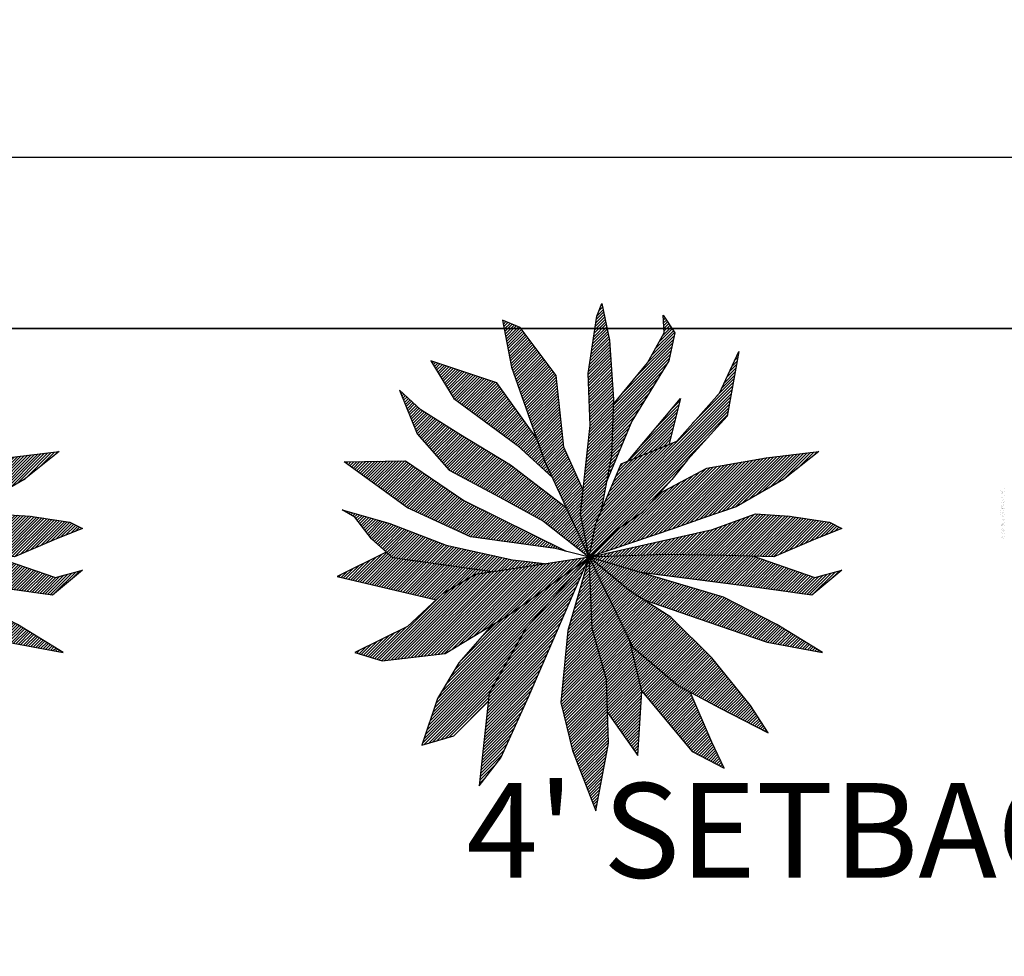
# Model space of a CAD drawing. Units: inches. Extents: x 1986 to 21484, y -1816 to 2016.
# Tile 10 of 85: x 2076 to 2149, y 1854 to 1924. Entities that reach past the tile are written whole.
import ezdxf

# ---------------------------------------------------------------- set-up
doc = ezdxf.new("R2010")
doc.units = ezdxf.units.IN
for name, color, linetype, lineweight in [('A-ANNO-DIMS', 2, 'Continuous', 18), ('A-ANNO-TEXT', 7, 'Continuous', 18), ('C-PROP', 7, 'Continuous', 35), ('L-PLNT', 84, 'Continuous', 13), ('vfolhas', 114, 'Continuous', 5)]:
    doc.layers.add(name, color=color, linetype=linetype, lineweight=lineweight)
for name, color, linetype in [('vfolha', 72, 'Continuous'), ('vfolha2', 110, 'Continuous'), ('vfolhas2', 102, 'Continuous')]:
    doc.layers.add(name, color=color, linetype=linetype)
doc.styles.get("Standard").update_dxf_attribs({"font": 'arial.ttf'})
doc.dimstyles.new('ISO-25', dxfattribs={"dimtxt": 8, "dimasz": 2.5, "dimexe": 1.25, "dimexo": 0.625, "dimtad": 1, "dimdec": 1, "dimlunit": 3, "dimtxsty": 'Standard', "dimcen": 2.5, "dimadec": 0, "dimazin": 0, "dimtfac": 1, "dimtdec": 1, "dimtmove": 0, "dimatfit": 3, "dimfxl": 1, "dimarcsym": 0})
pattern_1 = [(45, (-2446.5133113, 50.986076), (-0.004419417382, 0.004419417382), [])]

# ---------------------------------------------------------------- blocks, each defined once
blk = doc.blocks.new('*D1')
at = {"layer": 'A-ANNO-DIMS', "color": 0, "lineweight": -2, "transparency": 16777216}
for p, q in [((2042.312, 1901.377), (2042.312, 1914.655)), ((2402.312, 1901.377), (2402.312, 1914.655)), ((2044.812, 1913.405), (2399.812, 1913.405))]:
    blk.add_line(p, q, dxfattribs=at)
at = {"layer": 'A-ANNO-DIMS', "color": 0, "transparency": 16777216}
for points in [[(2044.812, 1913.821), (2044.812, 1912.988), (2042.312, 1913.405)], [(2399.812, 1913.821), (2399.812, 1912.988), (2402.312, 1913.405)]]:
    blk.add_solid(points, dxfattribs=at)
at = {"layer": 'Defpoints', "color": 0, "transparency": 16777216}
for p in [(2402.312, 1913.405), (2042.312, 1900.752), (2402.312, 1900.752)]:
    blk.add_point(p, dxfattribs=at)
at = {"layer": 'A-ANNO-DIMS', "color": 0, "transparency": 16777216, "insert": (2222.312, 1918.117), "char_height": 8, "attachment_point": 5}
blk.add_mtext("30'", dxfattribs=at)
blk = doc.blocks.new('arbusto_PB_verde_grande')
at = {"layer": 'vfolha2'}
h = blk.add_hatch(dxfattribs=at)
h.set_pattern_fill('ANSI31', color=256, scale=0.05, style=0)
h.set_pattern_definition(pattern_1)
h.paths.add_polyline_path([(0.0294, 0.3565), (0.0003, 0.0905), (0.0263, -0.0393), (0.047, 0.0623), (0.0619, 0.0973), (0.0937, 0.2657), (0.0996, 0.4347), (0.0879, 0.6131), (0.0645, 0.7227), (0.0499, 0.6851), (0.0236, 0.5129)])
h.paths.add_polyline_path([(0.3011, 0.4379), (0.1423, 0.2487), (0.2669, 0.3002)])
h.paths.add_polyline_path([(0.38, 0.2282), (0.237, 0.1519), (0.1843, 0.0936), (0.1112, 0.0436), (0.0263, -0.0393), (0.2806, 0.0467), (0.3683, 0.078), (0.4676, 0.1124), (0.6107, 0.1938), (0.7159, 0.2782), (0.5581, 0.2595)])
h.paths.add_polyline_path([(0.561, -0.2944), (0.7275, -0.3257), (0.5902, -0.2412), (0.4296, -0.1598), (0.0263, -0.0393), (0.1492, -0.1411), (0.1884, -0.166), (0.415, -0.2444)])
h.paths.add_polyline_path([(-0.2743, -0.4478), (-0.3035, -0.7263), (-0.2392, -0.6417), (-0.1546, -0.4572), (0.0263, -0.0393), (-0.1633, -0.2538)])
h.paths.add_polyline_path([(-0.5196, -0.2474), (-0.6774, -0.3257), (-0.5956, -0.3507), (-0.4057, -0.3288), (-0.2101, -0.21), (0.0263, -0.0393), (-0.1487, -0.0659), (-0.3152, -0.091), (-0.4145, -0.1505)])
h.paths.add_polyline_path([(-0.5255, 0.2501), (-0.7095, 0.247), (-0.5196, 0.1093), (-0.3298, 0.0217), (-0.0757, -0.0128), (-0.0423, -0.0215), (-0.3502, 0.1312)])
h = blk.add_hatch(dxfattribs=at)
h.set_pattern_fill('ANSI31', color=256, scale=0.05, style=0)
h.set_pattern_definition(pattern_1)
h.paths.add_polyline_path([(-0.1896, 0.297), (-0.0855, 0.2019), (-0.1078, 0.2501), (-0.132, 0.3187), (-0.251, 0.4848), (-0.4495, 0.5505), (-0.3795, 0.4379)])
h.paths.add_polyline_path([(0.0791, -0.4071), (0.0821, -0.5063), (0.1726, -0.6355), (0.1843, -0.4415), (0.149, -0.2918), (0.0263, -0.0393), (0.0353, -0.2538)])
at = {"layer": 'vfolhas'}
h = blk.add_hatch(dxfattribs=at)
h.set_pattern_fill('ANSI31', color=256, scale=0.05, style=0)
h.set_pattern_definition(pattern_1)
h.paths.add_polyline_path([(-0.0728, 0.5067), (-0.1808, 0.6506), (-0.2334, 0.6725), (-0.2071, 0.5318), (-0.1078, 0.2501), (0.0263, -0.0393), (0.0003, 0.0905), (0.0082, 0.1624), (-0.0494, 0.2908)])
h.paths.add_polyline_path([(0.099, 0.4193), (0.0937, 0.2657), (0.0791, 0.1881), (0.1551, 0.369), (0.2661, 0.5505), (0.2836, 0.635), (0.2485, 0.6882), (0.2514, 0.635), (0.2018, 0.5443)])
h.paths.add_polyline_path([(0.1229, 0.2407), (0.047, 0.0623), (0.0263, -0.0393), (0.1112, 0.0436), (0.1843, 0.0936), (0.2748, 0.1938), (0.3215, 0.2532), (0.4413, 0.3847), (0.4763, 0.5787), (0.4179, 0.4535), (0.2894, 0.3095)])
h.paths.add_polyline_path([(0.5815, -0.0378), (0.7071, 0.0154), (0.7859, 0.0467), (0.748, 0.0655), (0.6282, 0.0842), (0.526, 0.0905), (0.3974, 0.0436), (0.0263, -0.0393), (0.2573, -0.0315), (0.4383, -0.0347)])
h.paths.add_polyline_path([(0.5202, -0.0365), (0.4383, -0.0347), (0.2573, -0.0315), (0.0263, -0.0393), (0.1796, -0.0852), (0.5377, -0.1317), (0.6954, -0.1536), (0.7859, -0.0785), (0.7041, -0.1004)])
h.paths.add_polyline_path([(0.2719, -0.2193), (0.1492, -0.1411), (0.0263, -0.0393), (0.1579, -0.3101), (0.2952, -0.4258), (0.4179, -0.4916), (0.564, -0.5667), (0.5114, -0.4853), (0.3946, -0.3414)])
h.paths.add_polyline_path([(-0.0582, -0.4759), (-0.0231, -0.6198), (0.047, -0.8013), (0.0849, -0.5979), (0.0791, -0.4071), (0.0353, -0.2538), (0.0263, -0.0393), (-0.0377, -0.26)])
h.paths.add_polyline_path([(-0.2422, 0.1405), (-0.1107, 0.0686), (0.0263, -0.0393), (-0.0423, 0.1087), (-0.2101, 0.2376), (-0.3649, 0.3314), (-0.4787, 0.4034), (-0.543, 0.4629), (-0.4904, 0.3314), (-0.3941, 0.2219)])
h = blk.add_hatch(dxfattribs=at)
h.set_pattern_fill('ANSI31', color=256, scale=0.05, style=0)
h.set_pattern_definition(pattern_1)
h.paths.add_polyline_path([(-0.5722, 0.0623), (-0.7153, 0.103), (-0.6774, 0.0811), (-0.6277, 0.0154), (-0.5635, -0.041), (-0.2646, -0.0834), (-0.1487, -0.0659), (-0.1015, -0.0588), (-0.2042, -0.0472), (-0.4028, -0.0034)])
h.paths.add_polyline_path([(-0.5635, -0.041), (-0.5828, -0.024), (-0.7299, -0.0973), (-0.4334, -0.1679), (-0.4145, -0.1505), (-0.3152, -0.091), (-0.2646, -0.0834)])
h.paths.add_polyline_path([(-0.2769, -0.4727), (-0.2743, -0.4478), (-0.1633, -0.2538), (0.0263, -0.0393), (-0.2101, -0.21), (-0.2672, -0.2447), (-0.3649, -0.357), (-0.4291, -0.4634), (-0.4759, -0.6043), (-0.3795, -0.576)])
h = blk.add_hatch(dxfattribs=at)
h.set_pattern_fill('ANSI31', color=256, scale=0.05, style=0)
h.set_pattern_definition(pattern_1)
h.paths.add_polyline_path([(0.3361, -0.623), (0.4325, -0.6731), (0.3946, -0.5948), (0.3303, -0.4446), (0.2952, -0.4258), (0.1579, -0.3101), (0.149, -0.2918), (0.1843, -0.4415)])
at = {"layer": 'vfolha'}
for p, q in [((0.0263, -0.0393), (-0.1487, -0.0659)), ((0.0263, -0.0393), (-0.0377, -0.26)), ((0.0353, -0.2538), (0.0263, -0.0393)), ((0.5202, -0.0365), (0.7041, -0.1004)), ((0.5377, -0.1317), (0.1796, -0.0852)), ((0.7859, -0.0785), (0.6954, -0.1536)), ((0.7041, -0.1004), (0.7859, -0.0785)), ((0.6954, -0.1536), (0.5377, -0.1317)), ((0.3946, -0.3414), (0.2719, -0.2193)), ((-0.2672, -0.2447), (-0.3649, -0.357)), ((-0.0377, -0.26), (-0.0582, -0.4759)), ((0.0791, -0.4071), (0.0353, -0.2538)), ((0.1579, -0.3101), (0.2952, -0.4258)), ((0.5114, -0.4853), (0.3946, -0.3414)), ((0.0849, -0.5979), (0.0791, -0.4071)), ((0.2952, -0.4258), (0.4179, -0.4916)), ((0.4179, -0.4916), (0.564, -0.5667)), ((0.564, -0.5667), (0.5114, -0.4853)), ((-0.0231, -0.6198), (0.047, -0.8013)), ((0.047, -0.8013), (0.0849, -0.5979))]:
    blk.add_line(p, q, dxfattribs=at)
at = {"layer": 'vfolha2'}
for p, q in [((0.0499, 0.6851), (0.0645, 0.7227)), ((0.0645, 0.7227), (0.0879, 0.6131)), ((0.0236, 0.5129), (0.0499, 0.6851)), ((0.0879, 0.6131), (0.0996, 0.4347)), ((-0.4495, 0.5505), (-0.3795, 0.4379)), ((-0.251, 0.4848), (-0.4495, 0.5505)), ((0.0294, 0.3565), (0.0236, 0.5129)), ((-0.132, 0.3187), (-0.251, 0.4848)), ((-0.3795, 0.4379), (-0.1896, 0.297)), ((0.0996, 0.4347), (0.0937, 0.2657)), ((0.1434, 0.2501), (0.3011, 0.4379)), ((0.3011, 0.4379), (0.2661, 0.297)), ((0.0003, 0.0905), (0.0294, 0.3565)), ((-0.1896, 0.297), (-0.0822, 0.1989)), ((0.5581, 0.2595), (0.7159, 0.2782)), ((0.7159, 0.2782), (0.6107, 0.1938)), ((-0.7095, 0.247), (-0.5255, 0.2501)), ((-0.5196, 0.1093), (-0.7095, 0.247)), ((-0.5255, 0.2501), (-0.3502, 0.1312)), ((0.38, 0.2282), (0.5581, 0.2595)), ((0.237, 0.1519), (0.38, 0.2282)), ((0.6107, 0.1938), (0.4676, 0.1124)), ((-0.3502, 0.1312), (-0.0423, -0.0215)), ((-0.3298, 0.0217), (-0.5196, 0.1093)), ((0.0263, -0.0393), (0.0003, 0.0905)), ((0.3683, 0.078), (0.2806, 0.0467)), ((0.2806, 0.0467), (0.0263, -0.0393)), ((-0.0757, -0.0128), (-0.3298, 0.0217)), ((-0.2101, -0.21), (0.0263, -0.0393)), ((0.0263, -0.0393), (-0.1633, -0.2538)), ((-0.1546, -0.4572), (0.0263, -0.0393)), ((0.4296, -0.1598), (0.0263, -0.0393)), ((0.0263, -0.0393), (0.1579, -0.3101)), ((-0.1487, -0.0659), (-0.3152, -0.091)), ((-0.3152, -0.091), (-0.4145, -0.1505)), ((-0.4145, -0.1505), (-0.5196, -0.2474)), ((0.1884, -0.166), (0.415, -0.2444)), ((0.5902, -0.2412), (0.4296, -0.1598)), ((-0.4057, -0.3288), (-0.2101, -0.21)), ((-0.5196, -0.2474), (-0.6774, -0.3257)), ((-0.1633, -0.2538), (-0.2743, -0.4478)), ((0.415, -0.2444), (0.561, -0.2944)), ((0.7275, -0.3257), (0.5902, -0.2412)), ((0.1843, -0.4415), (0.149, -0.2918)), ((0.561, -0.2944), (0.7275, -0.3257)), ((-0.6774, -0.3257), (-0.5956, -0.3507)), ((-0.5956, -0.3507), (-0.4057, -0.3288)), ((0.1726, -0.6355), (0.1843, -0.4415)), ((-0.2743, -0.4478), (-0.3035, -0.7263)), ((0.0821, -0.5063), (0.1726, -0.6355)), ((-0.3035, -0.7263), (-0.2392, -0.6417))]:
    blk.add_line(p, q, dxfattribs=at)
at = {"layer": 'vfolhas2'}
for p, q in [((0.2514, 0.635), (0.2485, 0.6882)), ((0.2485, 0.6882), (0.2836, 0.635)), ((-0.2334, 0.6725), (-0.2071, 0.5318)), ((-0.1808, 0.6506), (-0.2334, 0.6725)), ((-0.0728, 0.5067), (-0.1808, 0.6506)), ((0.2018, 0.5443), (0.2514, 0.635)), ((0.2836, 0.635), (0.2661, 0.5505)), ((0.4179, 0.4535), (0.4763, 0.5787)), ((0.4763, 0.5787), (0.4413, 0.3847)), ((0.099, 0.4193), (0.2018, 0.5443)), ((0.2661, 0.5505), (0.1551, 0.369)), ((-0.2071, 0.5318), (-0.1078, 0.2501)), ((-0.0494, 0.2908), (-0.0728, 0.5067)), ((-0.543, 0.4629), (-0.4904, 0.3314)), ((-0.4787, 0.4034), (-0.543, 0.4629)), ((0.2894, 0.3095), (0.4179, 0.4535)), ((-0.3649, 0.3314), (-0.4787, 0.4034)), ((0.4413, 0.3847), (0.3215, 0.2532)), ((0.1551, 0.369), (0.078, 0.1855)), ((-0.4904, 0.3314), (-0.3941, 0.2219)), ((-0.2101, 0.2376), (-0.3649, 0.3314)), ((0.1229, 0.2407), (0.2894, 0.3095)), ((0.0082, 0.1624), (-0.0494, 0.2908)), ((-0.0423, 0.1087), (-0.2101, 0.2376)), ((-0.1078, 0.2501), (0.0263, -0.0393)), ((0.047, 0.0623), (0.1229, 0.2407)), ((0.0937, 0.2657), (0.0619, 0.0973)), ((0.3215, 0.2532), (0.2748, 0.1938)), ((-0.3941, 0.2219), (-0.2422, 0.1405)), ((0.2748, 0.1938), (0.1843, 0.0936)), ((-0.2422, 0.1405), (-0.1107, 0.0686)), ((-0.6774, 0.0811), (-0.7153, 0.103)), ((-0.7153, 0.103), (-0.5722, 0.0623)), ((0.1843, 0.0936), (0.1112, 0.0436)), ((0.4676, 0.1124), (0.3683, 0.078)), ((0.3974, 0.0436), (0.526, 0.0905)), ((0.526, 0.0905), (0.6282, 0.0842)), ((-0.6277, 0.0154), (-0.6774, 0.0811)), ((-0.5722, 0.0623), (-0.4028, -0.0034)), ((-0.1107, 0.0686), (0.0263, -0.0393)), ((0.0263, -0.0393), (0.047, 0.0623)), ((0.6282, 0.0842), (0.748, 0.0655)), ((0.748, 0.0655), (0.7859, 0.0467)), ((0.0263, -0.0393), (0.3974, 0.0436)), ((0.1112, 0.0436), (0.0263, -0.0393)), ((0.7859, 0.0467), (0.7071, 0.0154)), ((-0.5635, -0.041), (-0.6277, 0.0154)), ((0.7071, 0.0154), (0.5815, -0.0378)), ((-0.5828, -0.024), (-0.7299, -0.0973)), ((-0.4028, -0.0034), (-0.2042, -0.0472)), ((0.0263, -0.0393), (-0.0757, -0.0128)), ((-0.2646, -0.0834), (-0.5635, -0.041)), ((-0.2042, -0.0472), (-0.0983, -0.0591)), ((0.2573, -0.0315), (0.0263, -0.0393)), ((0.1492, -0.1411), (0.0263, -0.0393)), ((0.4383, -0.0347), (0.2573, -0.0315)), ((0.5815, -0.0378), (0.4383, -0.0347)), ((-0.7299, -0.0973), (-0.4334, -0.1679)), ((0.2719, -0.2193), (0.1492, -0.1411)), ((-0.3649, -0.357), (-0.4291, -0.4634)), ((0.1843, -0.4415), (0.3361, -0.623)), ((0.3946, -0.5948), (0.329, -0.4417)), ((-0.4291, -0.4634), (-0.4759, -0.6043)), ((-0.3795, -0.576), (-0.2769, -0.4727)), ((-0.2392, -0.6417), (-0.1546, -0.4572)), ((-0.0582, -0.4759), (-0.0231, -0.6198)), ((-0.4759, -0.6043), (-0.3795, -0.576)), ((0.4325, -0.6731), (0.3946, -0.5948)), ((0.3361, -0.623), (0.4325, -0.6731))]:
    blk.add_line(p, q, dxfattribs=at)
blk = doc.blocks.new('PLANT-SHRUB')
for p, q in [((2148.383, 1888.758), (2148.383, 1888.758)), ((2148.429, 1888.695), (2148.429, 1888.695)), ((2148.432, 1888.53), (2148.432, 1888.53)), ((2148.437, 1888.684), (2148.437, 1888.684)), ((2148.494, 1888.273), (2148.494, 1888.273)), ((2148.497, 1888.622), (2148.497, 1888.622)), ((2148.497, 1888.513), (2148.497, 1888.513)), ((2148.512, 1888.684), (2148.512, 1888.684)), ((2148.527, 1888.649), (2148.527, 1888.649)), ((2148.625, 1888.382), (2148.625, 1888.382)), ((2148.626, 1888.913), (2148.626, 1888.913)), ((2148.635, 1888.69), (2148.635, 1888.69)), ((2148.402, 1887.606), (2148.402, 1887.606)), ((2148.412, 1887.914), (2148.412, 1887.914)), ((2148.412, 1887.914), (2148.412, 1887.914)), ((2148.422, 1888.222), (2148.422, 1888.222)), ((2148.426, 1887.514), (2148.426, 1887.514)), ((2148.438, 1887.677), (2148.438, 1887.677)), ((2148.491, 1888.036), (2148.491, 1888.036)), ((2148.494, 1887.556), (2148.494, 1887.556)), ((2148.555, 1887.914), (2148.555, 1887.914)), ((2148.564, 1887.85), (2148.564, 1887.85)), ((2148.574, 1887.641), (2148.574, 1887.641)), ((2148.604, 1887.766), (2148.604, 1887.766)), ((2148.614, 1888.074), (2148.614, 1888.074)), ((2148.623, 1887.957), (2148.623, 1887.957)), ((2148.381, 1886.99), (2148.381, 1886.99)), ((2148.386, 1887.144), (2148.386, 1887.144)), ((2148.391, 1887.298), (2148.391, 1887.298)), ((2148.417, 1887.455), (2148.417, 1887.455)), ((2148.469, 1886.855), (2148.469, 1886.855)), ((2148.476, 1887.441), (2148.476, 1887.441)), ((2148.478, 1886.91), (2148.478, 1886.91)), ((2148.483, 1887.033), (2148.483, 1887.033)), ((2148.5, 1887.444), (2148.5, 1887.444)), ((2148.5, 1887.112), (2148.5, 1887.112)), ((2148.505, 1887.468), (2148.505, 1887.468)), ((2148.574, 1886.842), (2148.574, 1886.842)), ((2148.584, 1887.15), (2148.584, 1887.15)), ((2148.594, 1887.458), (2148.594, 1887.458)), ((2148.607, 1887.311), (2148.607, 1887.311)), ((2148.628, 1887), (2148.628, 1887)), ((2148.63, 1887.427), (2148.63, 1887.427)), ((2148.399, 1886.189), (2148.399, 1886.189)), ((2148.405, 1886.215), (2148.405, 1886.215)), ((2148.454, 1886.26), (2148.454, 1886.26)), ((2148.473, 1886.257), (2148.473, 1886.257)), ((2148.483, 1886.287), (2148.483, 1886.287)), ((2148.488, 1886.204), (2148.488, 1886.204)), ((2148.53, 1886.612), (2148.53, 1886.612)), ((2148.537, 1886.312), (2148.537, 1886.312)), ((2148.552, 1886.61), (2148.552, 1886.61)), ((2148.554, 1886.226), (2148.554, 1886.226)), ((2148.564, 1886.534), (2148.564, 1886.534)), ((2148.604, 1886.355), (2148.604, 1886.355)), ((2148.618, 1886.187), (2148.618, 1886.187)), ((2148.622, 1886.414), (2148.622, 1886.414)), ((2148.635, 1886.599), (2148.635, 1886.599)), ((2148.408, 1885.911), (2148.408, 1885.911)), ((2148.448, 1885.673), (2148.448, 1885.673)), ((2148.471, 1885.792), (2148.471, 1885.792)), ((2148.475, 1885.954), (2148.475, 1885.954)), ((2148.534, 1885.61), (2148.534, 1885.61)), ((2148.54, 1885.369), (2148.54, 1885.369)), ((2148.544, 1885.918), (2148.544, 1885.918)), ((2148.589, 1885.709), (2148.589, 1885.709)), ((2148.607, 1885.819), (2148.607, 1885.819)), ((2148.624, 1885.358), (2148.624, 1885.358)), ((2148.63, 1885.605), (2148.63, 1885.605)), ((2148.636, 1885.846), (2148.636, 1885.846)), ((2148.46, 1885.308), (2148.46, 1885.308)), ((2148.524, 1885.302), (2148.524, 1885.302)), ((2148.6, 1885.233), (2148.6, 1885.233))]:
    blk.add_line(p, q)

msp = doc.modelspace()

# ---------------------------------------------------------------- linework, layer by layer
at = {"layer": 'C-PROP'}
msp.add_lwpolyline([(2042.312, 1900.752), (2402.312, 1900.752), (2402.312, 1066.752), (2042.312, 1066.752)], close=True, dxfattribs=at)

# ---------------------------------------------------------------- block references
at = {"layer": 'L-PLNT'}
msp.add_blockref('PLANT-SHRUB', (0, 0), dxfattribs=at)
at = {"layer": 'L-PLNT', "xscale": 24.60366729364114, "yscale": 24.60366729364114, "zscale": 24.60366729364114}
for p in [(2061.184, 1884.805), (2117.305, 1884.805)]:
    msp.add_blockref('arbusto_PB_verde_grande', p, dxfattribs=at)

# ---------------------------------------------------------------- texts
at = {"layer": 'A-ANNO-TEXT', "insert": (2108.883, 1867.143), "char_height": 7, "attachment_point": 1}
msp.add_mtext_dynamic_manual_height_columns("{\\fTimes New Roman|b0|i0|c0|p18;4' SETBACK}", width=105.61268, gutter_width=12.5, heights=[0], dxfattribs=at)

# ---------------------------------------------------------------- dimensions: what is measured, and where the dimension line sits
at = {"layer": 'A-ANNO-DIMS'}
dim = msp.add_linear_dim(base=(2402.312, 1913.405), p1=(2042.312, 1900.752), p2=(2402.312, 1900.752), dimstyle='ISO-25', override={"dimclrd": 0, "dimclre": 0, "dimclrt": 0}, dxfattribs=at)
dim.commit()
dim.dimension.update_dxf_attribs({"geometry": '*D1', "text_midpoint": (2222.312, 1918.117)})

doc.saveas('drawing.dxf')
